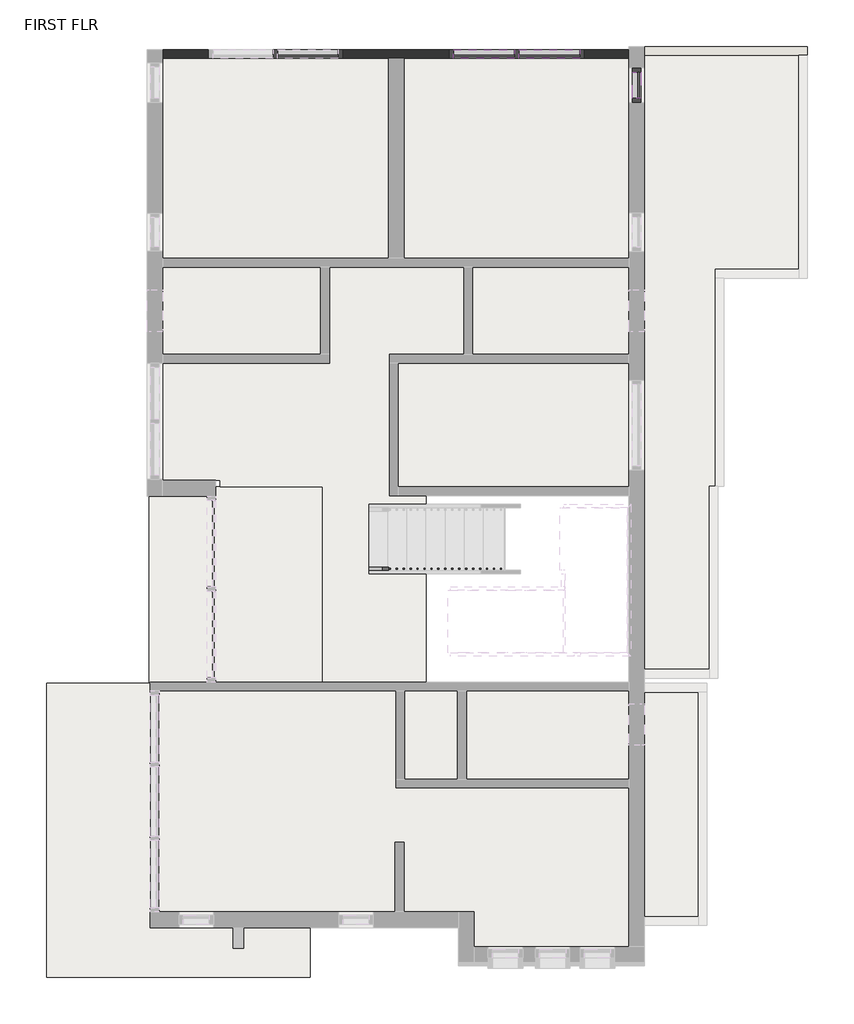
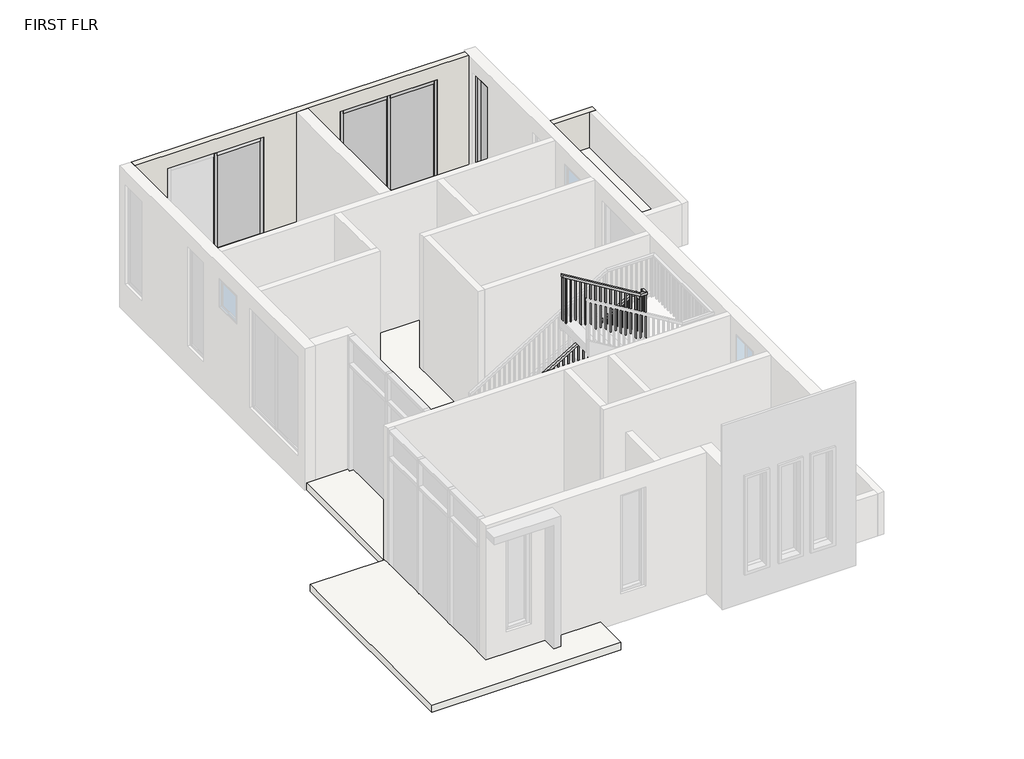
# One storey, part 3 of 4: 14 members, 4 plates, 2 slabs, 2 walls, 1 railing.
"""IFC4 building model written with IfcOpenShell, lengths in millimetres."""

from ifc_helpers import new_model, si_unit, frame, origin, place, context, project, spatial, polyline, outline, extrude, faceted_brep, transform, mapped, element, save
from components import member_dfe75557, member_3374d9b6, member_f1f71bde, member_5cd4c5ac, member_7cbddb58, system_panel_glazed_dc74cd20, system_panel_glazed_447bdfe9, system_panel_glazed_3ab3cb8c

model = new_model("IFC4")

# Units and contexts
model_context = context("Model", 3, world=origin())
ifc_project = project(units=[si_unit("LENGTHUNIT", "METRE", prefix="MILLI")], contexts=[model_context])

# Site, building, storey
site = spatial("IfcSite", under=ifc_project)
building = spatial("IfcBuilding", under=site)
storey = spatial("IfcBuildingStorey", under=building, Name="FIRST FLR", Elevation=3048.0)

# Members
placement = place(None, origin())
member_shape = member_dfe75557(model_context)
element("IfcMember", 1, ObjectType="Rectangular Mullion : 2.5\" x 5\" rectangular", at=placement, inside=storey, context=model_context, shape_type="MappedRepresentation", body=[
    mapped(member_shape, transform((-5795.8906521, 556.2983389, 5791.2), x_axis=(0.0, 0.0, 1.0), y_axis=(-1.0, 0.0, 0.0), z_axis=(0.0, -1.0, 0.0))),
])
element("IfcMember", 2, ObjectType="Rectangular Mullion : 2.5\" x 5\" rectangular", at=placement, inside=storey, context=model_context, shape_type="MappedRepresentation", body=[
    mapped(member_shape, transform((-5795.8906521, 937.2983389, 3657.6), x_axis=(0.0, 0.0, -1.0), y_axis=(-1.0, 0.0, 0.0), z_axis=(0.0, 1.0, 0.0))),
])
member_2_shape = member_3374d9b6(model_context)
element("IfcMember", 3, ObjectType="Rectangular Mullion : 2.5\" x 5\" rectangular", at=placement, inside=storey, context=model_context, shape_type="MappedRepresentation", body=[
    mapped(member_2_shape, transform((-5795.8906521, 492.7983389, 3657.6), x_axis=(0.0, -1.0, 0.0), y_axis=(-1.0, 0.0, 0.0), z_axis=(0.0, 0.0, -1.0))),
])
element("IfcMember", 4, ObjectType="Rectangular Mullion : 2.5\" x 5\" rectangular", at=placement, inside=storey, context=model_context, shape_type="MappedRepresentation", body=[
    mapped(member_2_shape, transform((-8539.0906521, 1203.9983389, 3657.6), x_axis=(-1.0, 0.0, 0.0), y_axis=(0.0, 1.0, 0.0), z_axis=(0.0, 0.0, -1.0))),
])
element("IfcMember", 5, ObjectType="Rectangular Mullion : 2.5\" x 5\" rectangular", at=placement, inside=storey, context=model_context, shape_type="MappedRepresentation", body=[
    mapped(member_2_shape, transform((-5795.8906521, 1000.7983389, 5791.2), x_axis=(0.0, 1.0, 0.0), y_axis=(-1.0, 0.0, 0.0), z_axis=(0.0, 0.0, 1.0))),
])
element("IfcMember", 6, ObjectType="Rectangular Mullion : 2.5\" x 5\" rectangular", at=placement, inside=storey, context=model_context, shape_type="MappedRepresentation", body=[
    mapped(member_2_shape, transform((-6557.8906521, 1203.9983389, 5791.2), x_axis=(1.0, 0.0, 0.0), y_axis=(0.0, 1.0, 0.0), z_axis=(0.0, 0.0, 1.0))),
])
element("IfcMember", 7, ObjectType="Rectangular Mullion : 2.5\" x 5\" rectangular", at=placement, inside=storey, context=model_context, shape_type="MappedRepresentation", body=[
    mapped(member_2_shape, transform((-10098.3911408, 1203.9983389, 5791.2), x_axis=(1.0, 0.0, 0.0), y_axis=(0.0, 1.0, 0.0), z_axis=(0.0, 0.0, 1.0))),
])
member_3_shape = member_f1f71bde(model_context)
element("IfcMember", 8, ObjectType="Rectangular Mullion : 2.5\" x 5\" rectangular", at=placement, inside=storey, context=model_context, shape_type="MappedRepresentation", body=[
    mapped(member_3_shape, transform((-8475.5906521, 1203.9983389, 5791.2), x_axis=(0.0, 0.0, 1.0), y_axis=(0.0, 1.0, 0.0), z_axis=(-1.0, 0.0, 0.0))),
])
element("IfcMember", 9, ObjectType="Rectangular Mullion : 2.5\" x 5\" rectangular", at=placement, inside=storey, context=model_context, shape_type="MappedRepresentation", body=[
    mapped(member_3_shape, transform((-7516.7406521, 1203.9983389, 5791.2), x_axis=(0.0, 0.0, 1.0), y_axis=(0.0, 1.0, 0.0), z_axis=(-1.0, 0.0, 0.0))),
])
element("IfcMember", 10, ObjectType="Rectangular Mullion : 2.5\" x 5\" rectangular", at=placement, inside=storey, context=model_context, shape_type="MappedRepresentation", body=[
    mapped(member_3_shape, transform((-6621.3906521, 1203.9983389, 3657.6), x_axis=(0.0, 0.0, -1.0), y_axis=(0.0, 1.0, 0.0), z_axis=(1.0, 0.0, 0.0))),
])
element("IfcMember", 11, ObjectType="Rectangular Mullion : 2.5\" x 5\" rectangular", at=placement, inside=storey, context=model_context, shape_type="MappedRepresentation", body=[
    mapped(member_3_shape, transform((-7580.2406521, 1203.9983389, 3657.6), x_axis=(0.0, 0.0, -1.0), y_axis=(0.0, 1.0, 0.0), z_axis=(1.0, 0.0, 0.0))),
])
member_4_shape = member_5cd4c5ac(model_context)
element("IfcMember", 12, ObjectType="Rectangular Mullion : 2.5\" x 5\" rectangular", at=placement, inside=storey, context=model_context, shape_type="MappedRepresentation", body=[
    mapped(member_4_shape, transform((-10161.8911408, 1203.9983389, 3657.6), x_axis=(0.0, 0.0, -1.0), y_axis=(0.0, 1.0, 0.0), z_axis=(1.0, 0.0, 0.0))),
])
member_5_shape = member_7cbddb58(model_context)
element("IfcMember", 13, ObjectType="Rectangular Mullion : 2.5\" x 5\" rectangular", at=placement, inside=storey, context=model_context, shape_type="MappedRepresentation", body=[
    mapped(member_5_shape, transform((-7548.4906521, 1203.9983389, 3657.6), x_axis=(-1.0, 0.0, 0.0), y_axis=(0.0, 1.0, 0.0), z_axis=(0.0, 0.0, -1.0))),
])
element("IfcMember", 14, ObjectType="Rectangular Mullion : 2.5\" x 5\" rectangular", at=placement, inside=storey, context=model_context, shape_type="MappedRepresentation", body=[
    mapped(member_5_shape, transform((-11076.2911408, 1203.9983389, 3657.6), x_axis=(-1.0, 0.0, 0.0), y_axis=(0.0, 1.0, 0.0), z_axis=(0.0, 0.0, -1.0))),
])

# Plates
system_panel_glazed_shape = system_panel_glazed_dc74cd20(model_context)
element("IfcPlate", 15, ObjectType="System Panel : Glazed", at=placement, inside=storey, context=model_context, shape_type="MappedRepresentation", body=[
    mapped(system_panel_glazed_shape, transform((-5795.8906521, 746.7983389, 3721.1), x_axis=(0.0, -1.0, 0.0), y_axis=(1.0, 0.0, 0.0), z_axis=(0.0, 0.0, 1.0))),
])
system_panel_glazed_2_shape = system_panel_glazed_447bdfe9(model_context)
element("IfcPlate", 16, ObjectType="System Panel : Glazed", at=placement, inside=storey, context=model_context, shape_type="MappedRepresentation", body=[
    mapped(system_panel_glazed_2_shape, transform((-7069.0656521, 1203.9983389, 3721.1), x_axis=(-1.0, 0.0, 0.0), y_axis=(0.0, -1.0, 0.0), z_axis=(0.0, 0.0, 1.0))),
])
element("IfcPlate", 17, ObjectType="System Panel : Glazed", at=placement, inside=storey, context=model_context, shape_type="MappedRepresentation", body=[
    mapped(system_panel_glazed_2_shape, transform((-8027.9156521, 1203.9983389, 3721.1), x_axis=(-1.0, 0.0, 0.0), y_axis=(0.0, -1.0, 0.0), z_axis=(0.0, 0.0, 1.0))),
])
system_panel_glazed_3_shape = system_panel_glazed_3ab3cb8c(model_context)
element("IfcPlate", 18, ObjectType="System Panel : Glazed", at=placement, inside=storey, context=model_context, shape_type="MappedRepresentation", body=[
    mapped(system_panel_glazed_3_shape, transform((-10603.2161408, 1203.9983389, 3721.1), x_axis=(-1.0, 0.0, 0.0), y_axis=(0.0, -1.0, 0.0), z_axis=(0.0, 0.0, 1.0))),
])

# Railing
element("IfcRailing", 19, ObjectType="Handrail - Rectangular", at=placement, inside=storey, context=model_context, shape_type="SolidModel", body=[
    faceted_brep([(-9709.3703437, -6296.9504041, 4131.7333333), (-9709.3703437, -6296.9504041, 4072.3318731), (-9709.3703437, -6347.7504041, 4072.3318731), (-9709.3703437, -6347.7504041, 4131.7333333), (-6915.3703437, -6296.9504041, 5825.0666667), (-6901.1779343, -6296.9504041, 5774.2666667), (-6901.1779343, -6347.7504041, 5774.2666667), (-6915.3703437, -6347.7504041, 5825.0666667), (-6790.5260609, -6296.9504041, 5825.0666667), (-6790.5260609, -6296.9504041, 5774.2666667), (-6841.3260609, -6347.7504041, 5774.2666667), (-6841.3260609, -6347.7504041, 5825.0666667), (-6790.5260609, -6562.8810793, 5825.0666667), (-6790.5260609, -6613.6810793, 5774.2666667), (-6841.3260609, -6613.6810793, 5774.2666667), (-6841.3260609, -6562.8810793, 5825.0666667), (-6790.5260609, -6562.8810793, 6040.5818182), (-6790.5260609, -6613.6810793, 5989.7818182), (-6841.3260609, -6613.6810793, 5989.7818182), (-6841.3260609, -6562.8810793, 6040.5818182), (-6790.5260609, -6689.8810793, 6040.5818182), (-6790.5260609, -6689.8810793, 5989.7818182), (-6841.3260609, -6639.0810793, 5989.7818182), (-6841.3260609, -6639.0810793, 6040.5818182), (-6917.5260609, -6689.8810793, 6040.5818182), (-6931.7184703, -6689.8810793, 5989.7818182), (-6931.7184703, -6639.0810793, 5989.7818182), (-6917.5260609, -6639.0810793, 6040.5818182), (-8517.7260609, -6689.8810793, 7010.4), (-8517.7260609, -6639.0810793, 7010.4), (-8517.7260609, -6639.0810793, 6950.9985397), (-8517.7260609, -6689.8810793, 6950.9985397)], [[[0, 1, 2, 3]], [[1, 0, 4, 5]], [[2, 1, 5, 6]], [[3, 2, 6, 7]], [[0, 3, 7, 4]], [[5, 4, 8, 9]], [[6, 5, 9, 10]], [[7, 6, 10, 11]], [[4, 7, 11, 8]], [[9, 8, 12, 13]], [[10, 9, 13, 14]], [[11, 10, 14, 15]], [[8, 11, 15, 12]], [[13, 12, 16, 17]], [[14, 13, 17, 18]], [[15, 14, 18, 19]], [[12, 15, 19, 16]], [[17, 16, 20, 21]], [[18, 17, 21, 22]], [[19, 18, 22, 23]], [[16, 19, 23, 20]], [[21, 20, 24, 25]], [[22, 21, 25, 26]], [[23, 22, 26, 27]], [[20, 23, 27, 24]], [[28, 29, 30, 31]], [[25, 24, 28, 31]], [[26, 25, 31, 30]], [[27, 26, 30, 29]], [[24, 27, 29, 28]]]),
    extrude(outline(polyline([(6899.0439943, -8432.0010609), (6910.5894488, -8451.0510609), (5926.6666667, -8451.0510609), (5926.6666667, -8432.0010609), (6899.0439943, -8432.0010609)])), frame((0.0, -6674.0060793, 0.0), z_axis=(0.0, 1.0, 0.0), x_axis=(0.0, 0.0, 1.0)), (0.0, 0.0, 1.0), 19.05),
    extrude(outline(polyline([(6837.4682367, -8330.4010609), (6849.0136913, -8349.4510609), (5926.6666667, -8349.4510609), (5926.6666667, -8330.4010609), (6837.4682367, -8330.4010609)])), frame((0.0, -6674.0060793, 0.0), z_axis=(0.0, 1.0, 0.0), x_axis=(0.0, 0.0, 1.0)), (0.0, 0.0, 1.0), 19.05),
    extrude(outline(polyline([(6775.8924791, -8228.8010609), (6787.4379337, -8247.8510609), (5926.6666667, -8247.8510609), (5926.6666667, -8228.8010609), (6775.8924791, -8228.8010609)])), frame((0.0, -6674.0060793, 0.0), z_axis=(0.0, 1.0, 0.0), x_axis=(0.0, 0.0, 1.0)), (0.0, 0.0, 1.0), 19.05),
    extrude(outline(polyline([(6714.3167216, -8127.2010609), (6725.8621761, -8146.2510609), (5757.3333333, -8146.2510609), (5757.3333333, -8127.2010609), (6714.3167216, -8127.2010609)])), frame((0.0, -6674.0060793, 0.0), z_axis=(0.0, 1.0, 0.0), x_axis=(0.0, 0.0, 1.0)), (0.0, 0.0, 1.0), 19.05),
    extrude(outline(polyline([(6652.740964, -8025.6010609), (6664.2864185, -8044.6510609), (5757.3333333, -8044.6510609), (5757.3333333, -8025.6010609), (6652.740964, -8025.6010609)])), frame((0.0, -6674.0060793, 0.0), z_axis=(0.0, 1.0, 0.0), x_axis=(0.0, 0.0, 1.0)), (0.0, 0.0, 1.0), 19.05),
    extrude(outline(polyline([(6591.1652064, -7924.0010609), (6602.710661, -7943.0510609), (5588.0, -7943.0510609), (5588.0, -7924.0010609), (6591.1652064, -7924.0010609)])), frame((0.0, -6674.0060793, 0.0), z_axis=(0.0, 1.0, 0.0), x_axis=(0.0, 0.0, 1.0)), (0.0, 0.0, 1.0), 19.05),
    extrude(outline(polyline([(6529.5894488, -7822.4010609), (6541.1349034, -7841.4510609), (5588.0, -7841.4510609), (5588.0, -7822.4010609), (6529.5894488, -7822.4010609)])), frame((0.0, -6674.0060793, 0.0), z_axis=(0.0, 1.0, 0.0), x_axis=(0.0, 0.0, 1.0)), (0.0, 0.0, 1.0), 19.05),
    extrude(outline(polyline([(6468.0136913, -7720.8010609), (6479.5591458, -7739.8510609), (5588.0, -7739.8510609), (5588.0, -7720.8010609), (6468.0136913, -7720.8010609)])), frame((0.0, -6674.0060793, 0.0), z_axis=(0.0, 1.0, 0.0), x_axis=(0.0, 0.0, 1.0)), (0.0, 0.0, 1.0), 19.05),
    extrude(outline(polyline([(6406.4379337, -7619.2010609), (6417.9833882, -7638.2510609), (5418.6666667, -7638.2510609), (5418.6666667, -7619.2010609), (6406.4379337, -7619.2010609)])), frame((0.0, -6674.0060793, 0.0), z_axis=(0.0, 1.0, 0.0), x_axis=(0.0, 0.0, 1.0)), (0.0, 0.0, 1.0), 19.05),
    extrude(outline(polyline([(6344.8621761, -7517.6010609), (6356.4076307, -7536.6510609), (5418.6666667, -7536.6510609), (5418.6666667, -7517.6010609), (6344.8621761, -7517.6010609)])), frame((0.0, -6674.0060793, 0.0), z_axis=(0.0, 1.0, 0.0), x_axis=(0.0, 0.0, 1.0)), (0.0, 0.0, 1.0), 19.05),
    extrude(outline(polyline([(6283.2864185, -7416.0010609), (6294.8318731, -7435.0510609), (5418.6666667, -7435.0510609), (5418.6666667, -7416.0010609), (6283.2864185, -7416.0010609)])), frame((0.0, -6674.0060793, 0.0), z_axis=(0.0, 1.0, 0.0), x_axis=(0.0, 0.0, 1.0)), (0.0, 0.0, 1.0), 19.05),
    extrude(outline(polyline([(6221.710661, -7314.4010609), (6233.2561155, -7333.4510609), (5249.3333333, -7333.4510609), (5249.3333333, -7314.4010609), (6221.710661, -7314.4010609)])), frame((0.0, -6674.0060793, 0.0), z_axis=(0.0, 1.0, 0.0), x_axis=(0.0, 0.0, 1.0)), (0.0, 0.0, 1.0), 19.05),
    extrude(outline(polyline([(6160.1349034, -7212.8010609), (6171.6803579, -7231.8510609), (5249.3333333, -7231.8510609), (5249.3333333, -7212.8010609), (6160.1349034, -7212.8010609)])), frame((0.0, -6674.0060793, 0.0), z_axis=(0.0, 1.0, 0.0), x_axis=(0.0, 0.0, 1.0)), (0.0, 0.0, 1.0), 19.05),
    extrude(outline(polyline([(6098.5591458, -7111.2010609), (6110.1046004, -7130.2510609), (5249.3333333, -7130.2510609), (5249.3333333, -7111.2010609), (6098.5591458, -7111.2010609)])), frame((0.0, -6674.0060793, 0.0), z_axis=(0.0, 1.0, 0.0), x_axis=(0.0, 0.0, 1.0)), (0.0, 0.0, 1.0), 19.05),
    extrude(outline(polyline([(6036.9833882, -7009.6010609), (6048.5288428, -7028.6510609), (5080.0, -7028.6510609), (5080.0, -7009.6010609), (6036.9833882, -7009.6010609)])), frame((0.0, -6674.0060793, 0.0), z_axis=(0.0, 1.0, 0.0), x_axis=(0.0, 0.0, 1.0)), (0.0, 0.0, 1.0), 19.05),
    extrude(outline(polyline([(5975.4076307, -6908.0010609), (5986.9530852, -6927.0510609), (5080.0, -6927.0510609), (5080.0, -6908.0010609), (5975.4076307, -6908.0010609)])), frame((0.0, -6674.0060793, 0.0), z_axis=(0.0, 1.0, 0.0), x_axis=(0.0, 0.0, 1.0)), (0.0, 0.0, 1.0), 19.05),
    extrude(outline(polyline([(-6825.4510609, -6617.6254041), (-6806.4010609, -6617.6254041), (-6806.4010609, -6636.6754041), (-6825.4510609, -6636.6754041), (-6825.4510609, -6617.6254041)])), frame((0.0, 0.0, 4910.6666667), z_axis=(0.0, 0.0, 1.0), x_axis=(1.0, 0.0, 0.0)), (0.0, 0.0, 1.0), 1079.1151515),
    extrude(outline(polyline([(-6825.4510609, -6516.0254041), (-6806.4010609, -6516.0254041), (-6806.4010609, -6535.0754041), (-6825.4510609, -6535.0754041), (-6825.4510609, -6516.0254041)])), frame((0.0, 0.0, 4910.6666667), z_axis=(0.0, 0.0, 1.0), x_axis=(1.0, 0.0, 0.0)), (0.0, 0.0, 1.0), 863.6),
    extrude(outline(polyline([(-6825.4510609, -6414.4254041), (-6806.4010609, -6414.4254041), (-6806.4010609, -6433.4754041), (-6825.4510609, -6433.4754041), (-6825.4510609, -6414.4254041)])), frame((0.0, 0.0, 4910.6666667), z_axis=(0.0, 0.0, 1.0), x_axis=(1.0, 0.0, 0.0)), (0.0, 0.0, 1.0), 863.6),
    extrude(outline(polyline([(5740.6500549, -6956.6453437), (5729.1046004, -6975.6953437), (4741.3333333, -6975.6953437), (4741.3333333, -6956.6453437), (5740.6500549, -6956.6453437)])), frame((0.0, -6331.8754041, 0.0), z_axis=(0.0, 1.0, 0.0), x_axis=(0.0, 0.0, 1.0)), (0.0, 0.0, 1.0), 19.05),
    extrude(outline(polyline([(5679.0742973, -7058.2453437), (5667.5288428, -7077.2953437), (4741.3333333, -7077.2953437), (4741.3333333, -7058.2453437), (5679.0742973, -7058.2453437)])), frame((0.0, -6331.8754041, 0.0), z_axis=(0.0, 1.0, 0.0), x_axis=(0.0, 0.0, 1.0)), (0.0, 0.0, 1.0), 19.05),
    extrude(outline(polyline([(5617.4985397, -7159.8453437), (5605.9530852, -7178.8953437), (4741.3333333, -7178.8953437), (4741.3333333, -7159.8453437), (5617.4985397, -7159.8453437)])), frame((0.0, -6331.8754041, 0.0), z_axis=(0.0, 1.0, 0.0), x_axis=(0.0, 0.0, 1.0)), (0.0, 0.0, 1.0), 19.05),
    extrude(outline(polyline([(5555.9227822, -7261.4453437), (5544.3773276, -7280.4953437), (4572.0, -7280.4953437), (4572.0, -7261.4453437), (5555.9227822, -7261.4453437)])), frame((0.0, -6331.8754041, 0.0), z_axis=(0.0, 1.0, 0.0), x_axis=(0.0, 0.0, 1.0)), (0.0, 0.0, 1.0), 19.05),
    extrude(outline(polyline([(5494.3470246, -7363.0453437), (5482.80157, -7382.0953437), (4572.0, -7382.0953437), (4572.0, -7363.0453437), (5494.3470246, -7363.0453437)])), frame((0.0, -6331.8754041, 0.0), z_axis=(0.0, 1.0, 0.0), x_axis=(0.0, 0.0, 1.0)), (0.0, 0.0, 1.0), 19.05),
    extrude(outline(polyline([(5432.771267, -7464.6453437), (5421.2258125, -7483.6953437), (4572.0, -7483.6953437), (4572.0, -7464.6453437), (5432.771267, -7464.6453437)])), frame((0.0, -6331.8754041, 0.0), z_axis=(0.0, 1.0, 0.0), x_axis=(0.0, 0.0, 1.0)), (0.0, 0.0, 1.0), 19.05),
    extrude(outline(polyline([(5371.1955094, -7566.2453437), (5359.6500549, -7585.2953437), (4402.6666667, -7585.2953437), (4402.6666667, -7566.2453437), (5371.1955094, -7566.2453437)])), frame((0.0, -6331.8754041, 0.0), z_axis=(0.0, 1.0, 0.0), x_axis=(0.0, 0.0, 1.0)), (0.0, 0.0, 1.0), 19.05),
    extrude(outline(polyline([(5309.6197519, -7667.8453437), (5298.0742973, -7686.8953437), (4402.6666667, -7686.8953437), (4402.6666667, -7667.8453437), (5309.6197519, -7667.8453437)])), frame((0.0, -6331.8754041, 0.0), z_axis=(0.0, 1.0, 0.0), x_axis=(0.0, 0.0, 1.0)), (0.0, 0.0, 1.0), 19.05),
    extrude(outline(polyline([(5248.0439943, -7769.4453437), (5236.4985397, -7788.4953437), (4233.3333333, -7788.4953437), (4233.3333333, -7769.4453437), (5248.0439943, -7769.4453437)])), frame((0.0, -6331.8754041, 0.0), z_axis=(0.0, 1.0, 0.0), x_axis=(0.0, 0.0, 1.0)), (0.0, 0.0, 1.0), 19.05),
    extrude(outline(polyline([(5186.4682367, -7871.0453437), (5174.9227822, -7890.0953437), (4233.3333333, -7890.0953437), (4233.3333333, -7871.0453437), (5186.4682367, -7871.0453437)])), frame((0.0, -6331.8754041, 0.0), z_axis=(0.0, 1.0, 0.0), x_axis=(0.0, 0.0, 1.0)), (0.0, 0.0, 1.0), 19.05),
    extrude(outline(polyline([(5124.8924791, -7972.6453437), (5113.3470246, -7991.6953437), (4233.3333333, -7991.6953437), (4233.3333333, -7972.6453437), (5124.8924791, -7972.6453437)])), frame((0.0, -6331.8754041, 0.0), z_axis=(0.0, 1.0, 0.0), x_axis=(0.0, 0.0, 1.0)), (0.0, 0.0, 1.0), 19.05),
    extrude(outline(polyline([(5063.3167216, -8074.2453437), (5051.771267, -8093.2953437), (4064.0, -8093.2953437), (4064.0, -8074.2453437), (5063.3167216, -8074.2453437)])), frame((0.0, -6331.8754041, 0.0), z_axis=(0.0, 1.0, 0.0), x_axis=(0.0, 0.0, 1.0)), (0.0, 0.0, 1.0), 19.05),
    extrude(outline(polyline([(5001.740964, -8175.8453437), (4990.1955094, -8194.8953437), (4064.0, -8194.8953437), (4064.0, -8175.8453437), (5001.740964, -8175.8453437)])), frame((0.0, -6331.8754041, 0.0), z_axis=(0.0, 1.0, 0.0), x_axis=(0.0, 0.0, 1.0)), (0.0, 0.0, 1.0), 19.05),
    extrude(outline(polyline([(4940.1652064, -8277.4453437), (4928.6197519, -8296.4953437), (4064.0, -8296.4953437), (4064.0, -8277.4453437), (4940.1652064, -8277.4453437)])), frame((0.0, -6331.8754041, 0.0), z_axis=(0.0, 1.0, 0.0), x_axis=(0.0, 0.0, 1.0)), (0.0, 0.0, 1.0), 19.05),
    extrude(outline(polyline([(4878.5894488, -8379.0453437), (4867.0439943, -8398.0953437), (3894.6666667, -8398.0953437), (3894.6666667, -8379.0453437), (4878.5894488, -8379.0453437)])), frame((0.0, -6331.8754041, 0.0), z_axis=(0.0, 1.0, 0.0), x_axis=(0.0, 0.0, 1.0)), (0.0, 0.0, 1.0), 19.05),
    extrude(outline(polyline([(4817.0136913, -8480.6453437), (4805.4682367, -8499.6953437), (3894.6666667, -8499.6953437), (3894.6666667, -8480.6453437), (4817.0136913, -8480.6453437)])), frame((0.0, -6331.8754041, 0.0), z_axis=(0.0, 1.0, 0.0), x_axis=(0.0, 0.0, 1.0)), (0.0, 0.0, 1.0), 19.05),
    extrude(outline(polyline([(4755.4379337, -8582.2453437), (4743.8924791, -8601.2953437), (3894.6666667, -8601.2953437), (3894.6666667, -8582.2453437), (4755.4379337, -8582.2453437)])), frame((0.0, -6331.8754041, 0.0), z_axis=(0.0, 1.0, 0.0), x_axis=(0.0, 0.0, 1.0)), (0.0, 0.0, 1.0), 19.05),
    extrude(outline(polyline([(4693.8621761, -8683.8453437), (4682.3167216, -8702.8953437), (3725.3333333, -8702.8953437), (3725.3333333, -8683.8453437), (4693.8621761, -8683.8453437)])), frame((0.0, -6331.8754041, 0.0), z_axis=(0.0, 1.0, 0.0), x_axis=(0.0, 0.0, 1.0)), (0.0, 0.0, 1.0), 19.05),
    extrude(outline(polyline([(4632.2864185, -8785.4453437), (4620.740964, -8804.4953437), (3725.3333333, -8804.4953437), (3725.3333333, -8785.4453437), (4632.2864185, -8785.4453437)])), frame((0.0, -6331.8754041, 0.0), z_axis=(0.0, 1.0, 0.0), x_axis=(0.0, 0.0, 1.0)), (0.0, 0.0, 1.0), 19.05),
    extrude(outline(polyline([(4570.710661, -8887.0453437), (4559.1652064, -8906.0953437), (3556.0, -8906.0953437), (3556.0, -8887.0453437), (4570.710661, -8887.0453437)])), frame((0.0, -6331.8754041, 0.0), z_axis=(0.0, 1.0, 0.0), x_axis=(0.0, 0.0, 1.0)), (0.0, 0.0, 1.0), 19.05),
    extrude(outline(polyline([(4509.1349034, -8988.6453437), (4497.5894488, -9007.6953437), (3556.0, -9007.6953437), (3556.0, -8988.6453437), (4509.1349034, -8988.6453437)])), frame((0.0, -6331.8754041, 0.0), z_axis=(0.0, 1.0, 0.0), x_axis=(0.0, 0.0, 1.0)), (0.0, 0.0, 1.0), 19.05),
    extrude(outline(polyline([(4447.5591458, -9090.2453437), (4436.0136913, -9109.2953437), (3556.0, -9109.2953437), (3556.0, -9090.2453437), (4447.5591458, -9090.2453437)])), frame((0.0, -6331.8754041, 0.0), z_axis=(0.0, 1.0, 0.0), x_axis=(0.0, 0.0, 1.0)), (0.0, 0.0, 1.0), 19.05),
    extrude(outline(polyline([(4385.9833882, -9191.8453437), (4374.4379337, -9210.8953437), (3386.6666667, -9210.8953437), (3386.6666667, -9191.8453437), (4385.9833882, -9191.8453437)])), frame((0.0, -6331.8754041, 0.0), z_axis=(0.0, 1.0, 0.0), x_axis=(0.0, 0.0, 1.0)), (0.0, 0.0, 1.0), 19.05),
    extrude(outline(polyline([(4324.4076307, -9293.4453437), (4312.8621761, -9312.4953437), (3386.6666667, -9312.4953437), (3386.6666667, -9293.4453437), (4324.4076307, -9293.4453437)])), frame((0.0, -6331.8754041, 0.0), z_axis=(0.0, 1.0, 0.0), x_axis=(0.0, 0.0, 1.0)), (0.0, 0.0, 1.0), 19.05),
    extrude(outline(polyline([(4262.8318731, -9395.0453437), (4251.2864185, -9414.0953437), (3386.6666667, -9414.0953437), (3386.6666667, -9395.0453437), (4262.8318731, -9395.0453437)])), frame((0.0, -6331.8754041, 0.0), z_axis=(0.0, 1.0, 0.0), x_axis=(0.0, 0.0, 1.0)), (0.0, 0.0, 1.0), 19.05),
    extrude(outline(polyline([(4201.2561155, -9496.6453437), (4189.710661, -9515.6953437), (3217.3333333, -9515.6953437), (3217.3333333, -9496.6453437), (4201.2561155, -9496.6453437)])), frame((0.0, -6331.8754041, 0.0), z_axis=(0.0, 1.0, 0.0), x_axis=(0.0, 0.0, 1.0)), (0.0, 0.0, 1.0), 19.05),
    extrude(outline(polyline([(4139.6803579, -9598.2453437), (4128.1349034, -9617.2953437), (3217.3333333, -9617.2953437), (3217.3333333, -9598.2453437), (4139.6803579, -9598.2453437)])), frame((0.0, -6331.8754041, 0.0), z_axis=(0.0, 1.0, 0.0), x_axis=(0.0, 0.0, 1.0)), (0.0, 0.0, 1.0), 19.05),
    extrude(outline(polyline([(-6825.4510609, -6654.9560793), (-6806.4010609, -6654.9560793), (-6806.4010609, -6674.0060793), (-6825.4510609, -6674.0060793), (-6825.4510609, -6654.9560793)])), frame((0.0, 0.0, 4910.6666667), z_axis=(0.0, 0.0, 1.0), x_axis=(1.0, 0.0, 0.0)), (0.0, 0.0, 1.0), 1079.1151515),
    extrude(outline(polyline([(-6825.4510609, -6331.8754041), (-6825.4510609, -6312.8254041), (-6806.4010609, -6312.8254041), (-6806.4010609, -6331.8754041), (-6825.4510609, -6331.8754041)])), frame((0.0, 0.0, 4910.6666667), z_axis=(0.0, 0.0, 1.0), x_axis=(1.0, 0.0, 0.0)), (0.0, 0.0, 1.0), 863.6),
    extrude(outline(polyline([(5771.4379337, -6905.8453437), (5759.8924791, -6924.8953437), (4910.6666667, -6924.8953437), (4910.6666667, -6905.8453437), (5771.4379337, -6905.8453437)])), frame((0.0, -6331.8754041, 0.0), z_axis=(0.0, 1.0, 0.0), x_axis=(0.0, 0.0, 1.0)), (0.0, 0.0, 1.0), 19.05),
    extrude(outline(polyline([(6939.4530852, -8498.6760609), (6950.9985397, -8517.7260609), (5926.6666667, -8517.7260609), (5926.6666667, -8498.6760609), (6939.4530852, -8498.6760609)])), frame((0.0, -6674.0060793, 0.0), z_axis=(0.0, 1.0, 0.0), x_axis=(0.0, 0.0, 1.0)), (0.0, 0.0, 1.0), 19.05),
    extrude(outline(polyline([(4083.8773276, -9690.3203437), (4072.3318731, -9709.3703437), (3217.3333333, -9709.3703437), (3217.3333333, -9690.3203437), (4083.8773276, -9690.3203437)])), frame((0.0, -6331.8754041, 0.0), z_axis=(0.0, 1.0, 0.0), x_axis=(0.0, 0.0, 1.0)), (0.0, 0.0, 1.0), 19.05),
])

# Slabs
element("IfcSlab", 20, ObjectType="MARBLE FLOORING 6\"", at=placement, inside=storey, context=model_context, shape_type="SweptSolid", body=[
    extrude(outline(polyline([(-9425.2911408, 1140.4983389), (-9425.2911408, -1785.0951712), (-12726.840556, -1785.0951712), (-12726.840556, 1140.4983389), (-9425.2911408, 1140.4983389)])), frame((0.0, 0.0, 3048.0), z_axis=(0.0, 0.0, 1.0), x_axis=(1.0, 0.0, 0.0)), (0.0, 0.0, 1.0), 152.4),
    extrude(outline(polyline([(-5910.1906521, 1140.4983389), (-5910.1906521, -1785.0951712), (-9196.6911408, -1785.0951712), (-9196.6911408, 1140.4983389), (-5910.1906521, 1140.4983389)])), frame((0.0, 0.0, 3048.0), z_axis=(0.0, 0.0, 1.0), x_axis=(1.0, 0.0, 0.0)), (0.0, 0.0, 1.0), 152.4),
    extrude(outline(polyline([(-10415.440556, -1912.0951712), (-10415.440556, -3188.4451712), (-12726.840556, -3188.4451712), (-12726.840556, -1912.0951712), (-10415.440556, -1912.0951712)])), frame((0.0, 0.0, 3048.0), z_axis=(0.0, 0.0, 1.0), x_axis=(1.0, 0.0, 0.0)), (0.0, 0.0, 1.0), 152.4),
    extrude(outline(polyline([(-5910.1906521, -1912.0951712), (-5910.1906521, -3188.4451712), (-8193.3911408, -3188.4451712), (-8193.3911408, -1912.0951712), (-5910.1906521, -1912.0951712)])), frame((0.0, 0.0, 3048.0), z_axis=(0.0, 0.0, 1.0), x_axis=(1.0, 0.0, 0.0)), (0.0, 0.0, 1.0), 152.4),
    extrude(outline(polyline([(-5910.1906521, -3315.4451712), (-5910.1906521, -5125.1951712), (-9282.0406521, -5125.1951712), (-9282.0406521, -3315.4451712), (-5910.1906521, -3315.4451712)])), frame((0.0, 0.0, 3048.0), z_axis=(0.0, 0.0, 1.0), x_axis=(1.0, 0.0, 0.0)), (0.0, 0.0, 1.0), 152.4),
    extrude(outline(polyline([(-8412.0906521, -8105.9310793), (-8412.0906521, -9397.5830995), (-9186.7906521, -9397.5830995), (-9186.7906521, -8105.9310793), (-8412.0906521, -8105.9310793)])), frame((0.0, 0.0, 3048.0), z_axis=(0.0, 0.0, 1.0), x_axis=(1.0, 0.0, 0.0)), (0.0, 0.0, 1.0), 152.4),
    extrude(outline(polyline([(-5910.1906521, -8105.9310793), (-5910.1906521, -9397.5830995), (-8285.0906521, -9397.5830995), (-8285.0906521, -8105.9310793), (-5910.1906521, -8105.9310793)])), frame((0.0, 0.0, 3048.0), z_axis=(0.0, 0.0, 1.0), x_axis=(1.0, 0.0, 0.0)), (0.0, 0.0, 1.0), 152.4),
    extrude(outline(polyline([(-14425.5406521, -12296.9310793), (-14425.5406521, -7997.9810793), (-12907.8906521, -7997.9810793), (-12907.8906521, -11568.2453012), (-10571.0906521, -11568.2453012), (-10571.0906521, -12296.9310793), (-14425.5406521, -12296.9310793)])), frame((0.0, 0.0, 3048.0), z_axis=(0.0, 0.0, 1.0), x_axis=(1.0, 0.0, 0.0)), (0.0, 0.0, 1.0), 152.4),
    extrude(outline(polyline([(-12780.8906521, -11339.6453012), (-12780.8906521, -8105.9310793), (-9313.7906521, -8105.9310793), (-9313.7906521, -9524.5830995), (-5910.1906521, -9524.5830995), (-5910.1906521, -11847.6453012), (-8170.7906521, -11847.6453012), (-8170.7906521, -11339.6453012), (-9199.4906521, -11339.6453012), (-9199.4906521, -10323.6453012), (-9326.4906521, -10323.6453012), (-9326.4906521, -11339.6453012), (-12780.8906521, -11339.6453012)])), frame((0.0, 0.0, 3048.0), z_axis=(0.0, 0.0, 1.0), x_axis=(1.0, 0.0, 0.0)), (0.0, 0.0, 1.0), 152.4),
    extrude(outline(polyline([(-4767.1906521, -7997.9810793), (-4767.1906521, -11534.9310793), (-5681.5906521, -11534.9310793), (-5681.5906521, -7997.9810793), (-4767.1906521, -7997.9810793)])), frame((0.0, 0.0, 3048.0), z_axis=(0.0, 0.0, 1.0), x_axis=(1.0, 0.0, 0.0)), (0.0, 0.0, 1.0), 152.4),
    extrude(outline(polyline([(-4732.5727979, -7921.7810793), (-5685.0727979, -7921.7810793), (-5685.0727979, 1311.7951326), (-3297.4727979, 1311.7951326), (-3297.4727979, -2071.8337491), (-4643.6727979, -2071.8337491), (-4643.6727979, -5119.6951024), (-4732.5727979, -5119.6951024), (-4732.5727979, -7921.7810793)])), frame((0.0, 0.0, 3048.0), z_axis=(0.0, 0.0, 1.0), x_axis=(1.0, 0.0, 0.0)), (0.0, 0.0, 1.0), 152.4),
    extrude(outline(polyline([(-10386.9406521, -7980.1161964), (-12920.5906521, -7980.1161964), (-12920.5906521, -5125.1951712), (-10386.9406521, -5125.1951712), (-10386.9406521, -7980.1161964)])), frame((0.0, 0.0, 3048.0), z_axis=(0.0, 0.0, 1.0), x_axis=(1.0, 0.0, 0.0)), (0.0, 0.0, 1.0), 152.4),
])
element("IfcSlab", 21, ObjectType="MARBLE FLOORING 6\"", at=placement, inside=storey, context=model_context, shape_type="SweptSolid", body=[
    extrude(outline(polyline([(-12726.840556, -3315.4451712), (-10288.440556, -3315.4451712), (-10288.440556, -1912.0951712), (-8320.3911408, -1912.0951712), (-8320.3911408, -3188.4451712), (-9409.0406521, -3188.4451712), (-9409.0406521, -5252.1951712), (-8875.6406521, -5252.1951712), (-8875.6406521, -5382.5504041), (-9709.3703437, -5382.5504041), (-9709.3703437, -6398.5504041), (-8875.6406521, -6398.5504041), (-8875.6406521, -7978.9310793), (-10323.4406521, -7978.9310793), (-10386.9406521, -7978.9310793), (-10386.9406521, -5125.1951712), (-11885.5406521, -5125.1951712), (-11885.5406521, -5031.7016611), (-12726.840556, -5031.7016611), (-12726.840556, -3315.4451712)])), frame((0.0, 0.0, 3048.0), z_axis=(0.0, 0.0, 1.0), x_axis=(1.0, 0.0, 0.0)), (0.0, 0.0, 1.0), 152.4),
])

# Walls
element("IfcWall", 22, ObjectType="INTERIOR WALL PAINT 5\"", at=placement, inside=storey, context=model_context, shape_type="Brep", body=[
    faceted_brep([(-12726.840556, 1140.4983389, 3048.0), (-9425.2911408, 1140.4983389, 3048.0), (-9196.6911408, 1140.4983389, 3048.0), (-5910.1906521, 1140.4983389, 3048.0), (-5910.1906521, 1140.4983389, 6096.0), (-9196.6911408, 1140.4983389, 6096.0), (-9425.2911408, 1140.4983389, 6096.0), (-12726.840556, 1140.4983389, 6096.0), (-6557.8906521, 1140.4983389, 5791.2), (-6557.8906521, 1140.4983389, 3657.6), (-8539.0906521, 1140.4983389, 3657.6), (-8539.0906521, 1140.4983389, 5791.2), (-10098.3911408, 1140.4983389, 5791.2), (-10098.3911408, 1140.4983389, 3657.6), (-12054.1911408, 1140.4983389, 3657.6), (-12054.1911408, 1140.4983389, 5791.2), (-5910.1906521, 1267.4983389, 3048.0), (-12726.840556, 1267.4983389, 3048.0), (-12726.840556, 1267.4983389, 6096.0), (-5910.1906521, 1267.4983389, 6096.0), (-6557.8906521, 1267.4983389, 3657.6), (-6557.8906521, 1267.4983389, 5791.2), (-8539.0906521, 1267.4983389, 5791.2), (-8539.0906521, 1267.4983389, 3657.6), (-10098.3911408, 1267.4983389, 3657.6), (-10098.3911408, 1267.4983389, 5791.2), (-12054.1911408, 1267.4983389, 5791.2), (-12054.1911408, 1267.4983389, 3657.6)], [[[0, 1, 2, 3, 4, 5, 6, 7], [8, 9, 10, 11], [12, 13, 14, 15]], [[16, 17, 18, 19], [20, 21, 22, 23], [24, 25, 26, 27]], [[3, 2, 1, 0, 17, 16]], [[7, 6, 5, 4, 19, 18]], [[0, 7, 18, 17]], [[4, 3, 16, 19]], [[8, 21, 20, 9]], [[21, 8, 11, 22]], [[22, 11, 10, 23]], [[9, 20, 23, 10]], [[24, 13, 12, 25]], [[25, 12, 15, 26]], [[26, 15, 14, 27]], [[13, 24, 27, 14]]]),
])
element("IfcWall", 23, ObjectType="INTERIOR WALL PAINT 5\"", at=placement, inside=storey, context=model_context, shape_type="Brep", body=[
    faceted_brep([(-5681.5906521, 1184.7951326, 3048.0), (-3424.4727979, 1184.7951326, 3048.0), (-3297.4727979, 1184.7951326, 3048.0), (-3297.4727979, 1184.7951326, 3962.4), (-3424.4727979, 1184.7951326, 3962.4), (-5681.5906521, 1184.7951326, 3962.4), (-5681.5906521, 1311.7951326, 3048.0), (-5681.5906521, 1311.7951326, 3962.4), (-3297.4727979, 1311.7951326, 3962.4), (-3297.4727979, 1311.7951326, 3048.0)], [[[0, 1, 2, 3, 4, 5]], [[6, 7, 8, 9]], [[2, 1, 0, 6, 9]], [[5, 4, 3, 8, 7]], [[0, 5, 7, 6]], [[3, 2, 9, 8]]]),
])

save(model, "model.ifc")

# Revit data of these elements
# Type "Rectangular Mullion : 2.5\" x 5\" rectangular"
#   built-in parameter 1007304 = 0.416667 (stored number, unit not read)
#   built-in parameter 1007301 = 0.104167 (stored number, unit not read)
#   built-in parameter 1007300 = 0.104167 (stored number, unit not read)
# Type "System Panel : Glazed"
#   Construction Type Id = "GSP4R"
#   Analytic Construction = "1/8 in Pilkington single glazing"
#   Visual Light Transmittance = 0.9
#   Solar Heat Gain Coefficient = 0.86
#   Heat Transfer Coefficient (U) = 1.18115 BTU/(h·ft²·°F)
#   Define Thermal Properties by = 1
# Type "Handrail - Rectangular"
#   Assembly Code = "C2010400"
#   built-in parameter 1008612 = 0.0416667 (stored number, unit not read)
#   built-in parameter 1008611 = 0.0416667 (stored number, unit not read)
#   built-in parameter 1008609 = 0.333333 (stored number, unit not read)
#   built-in parameter 1008604 = 0.166667 (stored number, unit not read)
#   built-in parameter 1008603 = 0.166667 (stored number, unit not read)
#   Railing Height = 3' - 0"
#   built-in parameter 1008630 = 2
#   built-in parameter 1008610 = 2
#   built-in parameter 1008618 = Baluster - Square : 3/4"
# Type "MARBLE FLOORING 6\""
#   Assembly Code = "B1010"
#   Function = 0
#   Layers, outside or top first: 0' - 6" "MARBLE FLOORING 1'" (function 1)
# Type "INTERIOR WALL PAINT 5\""
#   Assembly Code = "B2010"
#   Layers, outside or top first: 0' - 5" "EXTERIOR WALL PAINT" (function 1)
# Elements 1, 2, 3, 4, 5, 6, 7, 8, 9, 10, 11, 12, 13, 14 (IfcMember, "Rectangular Mullion : 2.5\" x 5\" rectangular")
#   Phase Created = New Construction
# Elements 15, 16, 17, 18 (IfcPlate, "System Panel : Glazed")
#   Phase Created = New Construction
#   Materials on its faces: "Glass"
# Element 19 (IfcRailing, "Handrail - Rectangular")
#   Phase Created = New Construction
# Element 20 (IfcSlab, "MARBLE FLOORING 6\"")
#   Height Offset From Level = 0' - 6"
#   Phase Created = New Construction
#   Materials on its faces: "MARBLE FLOORING 1'"
# Element 21 (IfcSlab, "MARBLE FLOORING 6\"")
#   built-in parameter 1001955 = 1.5708 (stored number, unit not read)
#   Height Offset From Level = 0' - 6"
#   Phase Created = New Construction
#   Materials on its faces: "MARBLE FLOORING 1'"
# Element 22 (IfcWall, "INTERIOR WALL PAINT 5\"")
#   Top Offset = 0' - 0"
#   Base Offset = 0' - 0"
#   wall height = 10' - 0"
#   Phase Created = New Construction
#   Base Constraint = FIRST FLR
#   Top Constraint = SECOND FLR
#   Materials on its faces: "EXTERIOR WALL PAINT"
# Element 23 (IfcWall, "INTERIOR WALL PAINT 5\"")
#   Top Offset = 0' - 0"
#   Base Offset = 0' - 0"
#   Unconnected Height = 3' - 0"
#   wall height = 3' - 0"
#   Phase Created = New Construction
#   Base Constraint = FIRST FLR
#   Materials on its faces: "EXTERIOR WALL PAINT"
# Materials
#   "MARBLE FLOORING 1'": class "Generic", colour RGB 120 120 120, transparency 0, Cost = 0
#   "EXTERIOR WALL PAINT": class "Generic", colour RGB 120 120 120, transparency 0, Cost = 0
#   "Glass": class "Glass", colour RGB 0 128 192, transparency 0.75, Description = "Soda Lime Glass", Cost = 0
